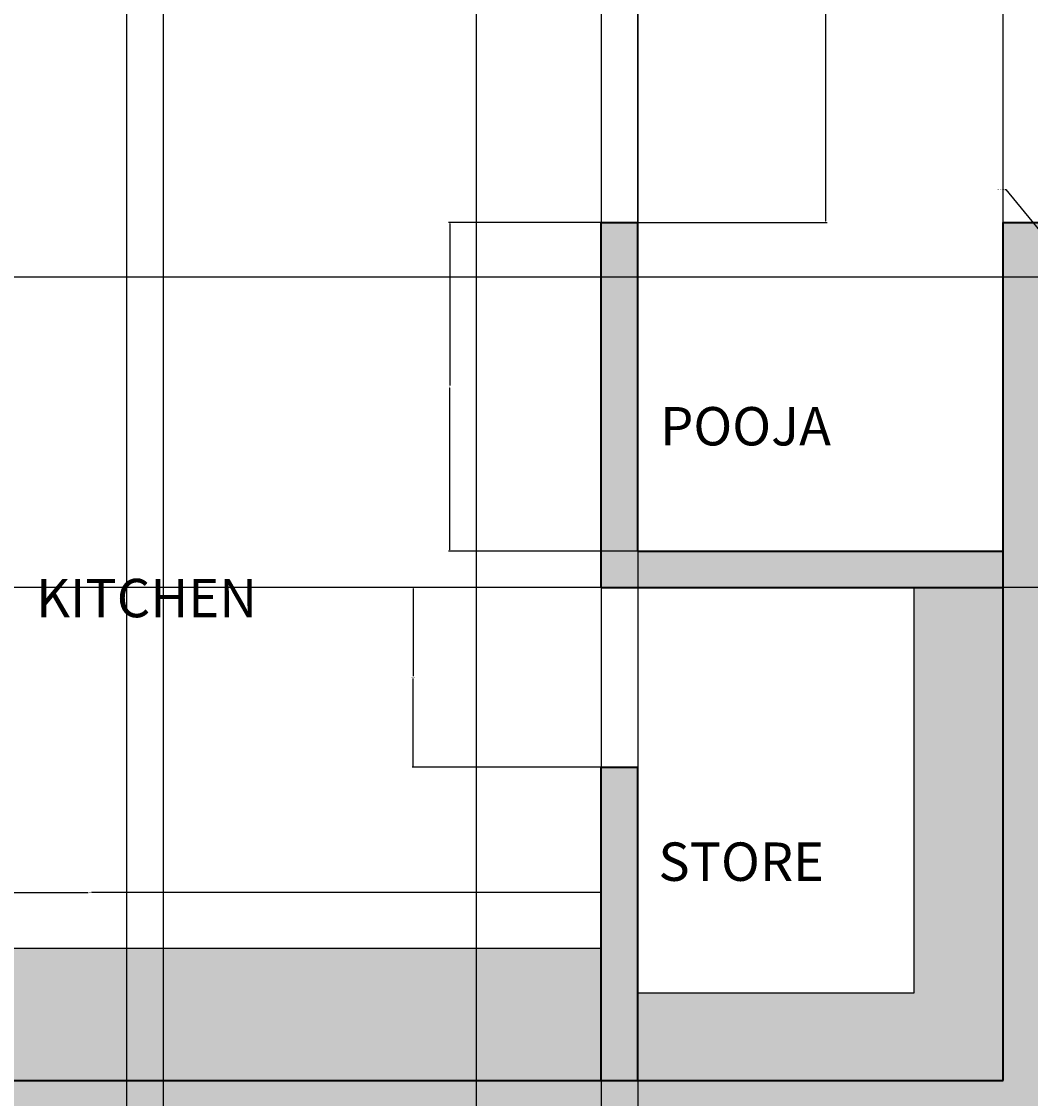
# Model space of a CAD drawing. Units: inches. Extents: x 2549 to 3108, y 1683 to 2362.
# Tile 3 of 30: x 2711 to 2877, y 1802 to 1979. Entities that reach past the tile are written whole.
import ezdxf

# ---------------------------------------------------------------- set-up
doc = ezdxf.new("R2010")
doc.units = ezdxf.units.IN
for name, color, linetype, lineweight in [('A-ANNO-DIMS', 2, 'Continuous', 18), ('A-AREA-IDEN', 7, 'Continuous', 18), ('A-FLOR-CASE', 8, 'Continuous', 25), ('A-FLOR-CASE-PATT', 42, 'Continuous', 13), ('A-FURN-PATT', 9, 'Continuous', 13), ('A-WALL', 7, 'Continuous', 35), ('A-WALL-PATT', 89, 'Continuous', 13)]:
    doc.layers.add(name, color=color, linetype=linetype, lineweight=lineweight)
doc.layers.add('C-PKNG-VEHI-PATT', color=251, linetype='Continuous', lineweight=13, true_color=0x636466)
doc.layers.add('C-PVMT-PATT', color=9, linetype='Continuous', lineweight=13, true_color=0xc7c8ca)
doc.styles.get("Standard").update_dxf_attribs({"font": 'arial.ttf'})
doc.dimstyles.get("Standard").update_dxf_attribs({"dimtxt": 0.18, "dimasz": 0.18, "dimexe": 0.18, "dimexo": 0.0625, "dimgap": 0.09, "dimtad": 0, "dimtih": 1, "dimtoh": 1, "dimdec": 4, "dimzin": 0, "dimdsep": 46, "dimtxsty": 'Standard', "dimcen": 0.09, "dimadec": 0, "dimazin": 0, "dimtfac": 1, "dimtdec": 4, "dimtofl": 0, "dimtmove": 0, "dimatfit": 3, "dimfxl": 1, "dimtolj": 1, "dimtzin": 0, "dimarcsym": 0})

# ---------------------------------------------------------------- blocks, each defined once
blk = doc.blocks.new('*D42')
at = {"layer": 'A-ANNO-DIMS', "color": 0, "lineweight": -2, "transparency": 16777216}
for p, q in [((2638.64, 2080.46), (2638.64, 1683.44)), ((2728.64, 2080.46), (2728.64, 1683.44)), ((2638.82, 1683.62), (2683.42, 1683.62)), ((2728.46, 1683.62), (2683.86, 1683.62))]:
    blk.add_line(p, q, dxfattribs=at)
at = {"layer": 'A-ANNO-DIMS', "color": 0, "transparency": 16777216}
for points in [[(2638.82, 1683.65), (2638.82, 1683.59), (2638.64, 1683.62)], [(2728.46, 1683.65), (2728.46, 1683.59), (2728.64, 1683.62)]]:
    blk.add_solid(points, dxfattribs=at)
at = {"layer": 'Defpoints', "color": 0, "transparency": 16777216}
for p in [(2638.64, 2080.52), (2728.64, 2080.52), (2728.64, 1683.62)]:
    blk.add_point(p, dxfattribs=at)
at = {"layer": 'A-ANNO-DIMS', "color": 0, "transparency": 16777216, "insert": (2683.64, 1683.62), "char_height": 0.18, "attachment_point": 5}
blk.add_mtext('\\A1;90', dxfattribs=at)
blk = doc.blocks.new('*D43')
at = {"layer": 'A-ANNO-DIMS', "color": 0, "lineweight": -2, "transparency": 16777216}
for p, q in [((2734.64, 2080.46), (2734.64, 1683.44)), ((2806.64, 2080.46), (2806.64, 1683.44)), ((2734.82, 1683.62), (2770.43, 1683.62)), ((2806.46, 1683.62), (2770.86, 1683.62))]:
    blk.add_line(p, q, dxfattribs=at)
at = {"layer": 'A-ANNO-DIMS', "color": 0, "transparency": 16777216}
for points in [[(2734.82, 1683.65), (2734.82, 1683.59), (2734.64, 1683.62)], [(2806.46, 1683.65), (2806.46, 1683.59), (2806.64, 1683.62)]]:
    blk.add_solid(points, dxfattribs=at)
at = {"layer": 'Defpoints', "color": 0, "transparency": 16777216}
for p in [(2734.64, 2080.52), (2806.64, 2080.52), (2806.64, 1683.62)]:
    blk.add_point(p, dxfattribs=at)
at = {"layer": 'A-ANNO-DIMS', "color": 0, "transparency": 16777216, "insert": (2770.64, 1683.62), "char_height": 0.18, "attachment_point": 5}
blk.add_mtext('\\A1;72', dxfattribs=at)
blk = doc.blocks.new('*D44')
at = {"layer": 'A-ANNO-DIMS', "color": 0, "lineweight": -2, "transparency": 16777216}
for p, q in [((2662.64, 2040.99), (2662.64, 1683.44)), ((2806.64, 2016.13), (2806.64, 1683.44)), ((2662.82, 1683.62), (2734.36, 1683.62)), ((2806.46, 1683.62), (2734.92, 1683.62))]:
    blk.add_line(p, q, dxfattribs=at)
at = {"layer": 'A-ANNO-DIMS', "color": 0, "transparency": 16777216}
for points in [[(2662.82, 1683.65), (2662.82, 1683.59), (2662.64, 1683.62)], [(2806.46, 1683.65), (2806.46, 1683.59), (2806.64, 1683.62)]]:
    blk.add_solid(points, dxfattribs=at)
at = {"layer": 'Defpoints', "color": 0, "transparency": 16777216}
for p in [(2662.64, 2041.06), (2806.64, 2016.19), (2806.64, 1683.62)]:
    blk.add_point(p, dxfattribs=at)
at = {"layer": 'A-ANNO-DIMS', "color": 0, "transparency": 16777216, "insert": (2734.64, 1683.62), "char_height": 0.18, "attachment_point": 5}
blk.add_mtext('\\A1;144', dxfattribs=at)
blk = doc.blocks.new('*D46')
at = {"layer": 'A-ANNO-DIMS', "color": 0, "lineweight": -2, "transparency": 16777216}
for p, q in [((2812.64, 2140.46), (2812.64, 1683.44)), ((3034.64, 2134.46), (3034.64, 1683.44)), ((2812.82, 1683.62), (2923.35, 1683.62)), ((3034.46, 1683.62), (2923.93, 1683.62))]:
    blk.add_line(p, q, dxfattribs=at)
at = {"layer": 'A-ANNO-DIMS', "color": 0, "transparency": 16777216}
for points in [[(2812.82, 1683.65), (2812.82, 1683.59), (2812.64, 1683.62)], [(3034.46, 1683.65), (3034.46, 1683.59), (3034.64, 1683.62)]]:
    blk.add_solid(points, dxfattribs=at)
at = {"layer": 'Defpoints', "color": 0, "transparency": 16777216}
for p in [(2812.64, 2140.52), (3034.64, 2134.52), (3034.64, 1683.62)]:
    blk.add_point(p, dxfattribs=at)
at = {"layer": 'A-ANNO-DIMS', "color": 0, "transparency": 16777216, "insert": (2923.64, 1683.62), "char_height": 0.18, "attachment_point": 5}
blk.add_mtext('\\A1;222', dxfattribs=at)
blk = doc.blocks.new('*D48')
at = {"layer": 'A-ANNO-DIMS', "color": 0, "lineweight": -2, "transparency": 16777216}
for p, q in [((2812.71, 2016.19), (2843.72, 2016.19)), ((2843.54, 2016.01), (2843.54, 1981.04)), ((2843.54, 1945.7), (2843.54, 1980.68)), ((2812.71, 1945.52), (2843.72, 1945.52))]:
    blk.add_line(p, q, dxfattribs=at)
at = {"layer": 'A-ANNO-DIMS', "color": 0, "transparency": 16777216}
for points in [[(2843.51, 2016.01), (2843.57, 2016.01), (2843.54, 2016.19)], [(2843.51, 1945.7), (2843.57, 1945.7), (2843.54, 1945.52)]]:
    blk.add_solid(points, dxfattribs=at)
at = {"layer": 'Defpoints', "color": 0, "transparency": 16777216}
for p in [(2812.64, 2016.19), (2812.64, 1945.52), (2843.54, 1945.52)]:
    blk.add_point(p, dxfattribs=at)
at = {"layer": 'A-ANNO-DIMS', "color": 0, "transparency": 16777216, "insert": (2843.54, 1980.86), "char_height": 0.18, "attachment_point": 5}
blk.add_mtext('\\A1;70.67', dxfattribs=at)
blk = doc.blocks.new('*D49')
at = {"layer": 'A-ANNO-DIMS', "color": 0, "lineweight": -2, "transparency": 16777216}
for p, q in [((2638.64, 1804.59), (2638.64, 1835.6)), ((2638.82, 1835.42), (2722.36, 1835.42)), ((2806.46, 1835.42), (2722.92, 1835.42)), ((2806.64, 1804.59), (2806.64, 1835.6))]:
    blk.add_line(p, q, dxfattribs=at)
at = {"layer": 'A-ANNO-DIMS', "color": 0, "transparency": 16777216}
for points in [[(2638.82, 1835.45), (2638.82, 1835.39), (2638.64, 1835.42)], [(2806.46, 1835.45), (2806.46, 1835.39), (2806.64, 1835.42)]]:
    blk.add_solid(points, dxfattribs=at)
at = {"layer": 'Defpoints', "color": 0, "transparency": 16777216}
for p in [(2806.64, 1835.42), (2638.64, 1804.52), (2806.64, 1804.52)]:
    blk.add_point(p, dxfattribs=at)
at = {"layer": 'A-ANNO-DIMS', "color": 0, "transparency": 16777216, "insert": (2722.64, 1835.42), "char_height": 0.18, "attachment_point": 5}
blk.add_mtext('\\A1;168', dxfattribs=at)
blk = doc.blocks.new('*D52')
at = {"layer": 'A-ANNO-DIMS', "color": 0, "lineweight": -2, "transparency": 16777216}
for p, q in [((2812.64, 1891.59), (2812.64, 2362.32)), ((2872.64, 1891.59), (2872.64, 2362.32)), ((2812.82, 2362.14), (2842.42, 2362.14)), ((2872.46, 2362.14), (2842.86, 2362.14))]:
    blk.add_line(p, q, dxfattribs=at)
at = {"layer": 'A-ANNO-DIMS', "color": 0, "transparency": 16777216}
for points in [[(2812.82, 2362.17), (2812.82, 2362.11), (2812.64, 2362.14)], [(2872.46, 2362.17), (2872.46, 2362.11), (2872.64, 2362.14)]]:
    blk.add_solid(points, dxfattribs=at)
at = {"layer": 'Defpoints', "color": 0, "transparency": 16777216}
for p in [(2872.64, 2362.14), (2812.64, 1891.52), (2872.64, 1891.52)]:
    blk.add_point(p, dxfattribs=at)
at = {"layer": 'A-ANNO-DIMS', "color": 0, "transparency": 16777216, "insert": (2842.64, 2362.14), "char_height": 0.18, "attachment_point": 5}
blk.add_mtext('\\A1;60', dxfattribs=at)
blk = doc.blocks.new('*D53')
at = {"layer": 'A-ANNO-DIMS', "color": 0, "lineweight": -2, "transparency": 16777216}
for p, q in [((2812.58, 1945.52), (2781.56, 1945.52)), ((2781.74, 1945.34), (2781.74, 1918.71)), ((2781.74, 1891.7), (2781.74, 1918.34)), ((2812.58, 1891.52), (2781.56, 1891.52))]:
    blk.add_line(p, q, dxfattribs=at)
at = {"layer": 'A-ANNO-DIMS', "color": 0, "transparency": 16777216}
for points in [[(2781.71, 1945.34), (2781.77, 1945.34), (2781.74, 1945.52)], [(2781.71, 1891.7), (2781.77, 1891.7), (2781.74, 1891.52)]]:
    blk.add_solid(points, dxfattribs=at)
at = {"layer": 'Defpoints', "color": 0, "transparency": 16777216}
for p in [(2781.74, 1945.52), (2812.64, 1945.52), (2812.64, 1891.52)]:
    blk.add_point(p, dxfattribs=at)
at = {"layer": 'A-ANNO-DIMS', "color": 0, "transparency": 16777216, "insert": (2781.74, 1918.52), "char_height": 0.18, "attachment_point": 5}
blk.add_mtext('\\A1;54', dxfattribs=at)
blk = doc.blocks.new('*D54')
at = {"layer": 'A-ANNO-DIMS', "color": 0, "lineweight": -2, "transparency": 16777216}
for p, q in [((2806.58, 1885.52), (2775.56, 1885.52)), ((2775.74, 1885.34), (2775.74, 1870.94)), ((2775.74, 1856.17), (2775.74, 1870.57)), ((2806.58, 1855.99), (2775.56, 1855.99))]:
    blk.add_line(p, q, dxfattribs=at)
at = {"layer": 'A-ANNO-DIMS', "color": 0, "transparency": 16777216}
for points in [[(2775.71, 1885.34), (2775.77, 1885.34), (2775.74, 1885.52)], [(2775.71, 1856.17), (2775.77, 1856.17), (2775.74, 1855.99)]]:
    blk.add_solid(points, dxfattribs=at)
at = {"layer": 'Defpoints', "color": 0, "transparency": 16777216}
for p in [(2775.74, 1885.52), (2806.64, 1885.52), (2806.64, 1855.99)]:
    blk.add_point(p, dxfattribs=at)
at = {"layer": 'A-ANNO-DIMS', "color": 0, "transparency": 16777216, "insert": (2775.74, 1870.75), "char_height": 0.18, "attachment_point": 5}
blk.add_mtext('\\A1;29.54', dxfattribs=at)
blk = doc.blocks.new('*D55')
at = {"layer": 'A-ANNO-DIMS', "color": 0, "lineweight": -2, "transparency": 16777216}
for p, q in [((2872.58, 1885.52), (2549.42, 1885.52)), ((2549.6, 1885.34), (2549.6, 1845.21)), ((2549.6, 1804.7), (2549.6, 1844.84)), ((2872.58, 1804.52), (2549.42, 1804.52))]:
    blk.add_line(p, q, dxfattribs=at)
at = {"layer": 'A-ANNO-DIMS', "color": 0, "transparency": 16777216}
for points in [[(2549.57, 1885.34), (2549.63, 1885.34), (2549.6, 1885.52)], [(2549.57, 1804.7), (2549.63, 1804.7), (2549.6, 1804.52)]]:
    blk.add_solid(points, dxfattribs=at)
at = {"layer": 'Defpoints', "color": 0, "transparency": 16777216}
for p in [(2549.6, 1885.52), (2872.64, 1885.52), (2872.64, 1804.52)]:
    blk.add_point(p, dxfattribs=at)
at = {"layer": 'A-ANNO-DIMS', "color": 0, "transparency": 16777216, "insert": (2549.6, 1845.02), "char_height": 0.18, "attachment_point": 5}
blk.add_mtext('\\A1;81', dxfattribs=at)
blk = doc.blocks.new('*D56')
at = {"layer": 'A-ANNO-DIMS', "color": 0, "lineweight": -2, "transparency": 16777216}
for p, q in [((3043.58, 1936.52), (2549.42, 1936.52)), ((2549.6, 1936.34), (2549.6, 1911.21)), ((2549.6, 1885.7), (2549.6, 1910.84)), ((3043.58, 1885.52), (2549.42, 1885.52))]:
    blk.add_line(p, q, dxfattribs=at)
at = {"layer": 'A-ANNO-DIMS', "color": 0, "transparency": 16777216}
for points in [[(2549.57, 1936.34), (2549.63, 1936.34), (2549.6, 1936.52)], [(2549.57, 1885.7), (2549.63, 1885.7), (2549.6, 1885.52)]]:
    blk.add_solid(points, dxfattribs=at)
at = {"layer": 'Defpoints', "color": 0, "transparency": 16777216}
for p in [(2549.6, 1936.52), (3043.64, 1936.52), (3043.64, 1885.52)]:
    blk.add_point(p, dxfattribs=at)
at = {"layer": 'A-ANNO-DIMS', "color": 0, "transparency": 16777216, "insert": (2549.6, 1911.02), "char_height": 0.18, "attachment_point": 5}
blk.add_mtext('\\A1;51', dxfattribs=at)
blk = doc.blocks.new('*D59')
at = {"layer": 'A-ANNO-DIMS', "color": 0, "lineweight": -2, "transparency": 16777216}
for p, q in [((2680.98, 1761.59), (2680.98, 2362.32)), ((2786.16, 1761.59), (2786.16, 2362.32)), ((2681.16, 2362.14), (2733.11, 2362.14)), ((2785.98, 2362.14), (2734.02, 2362.14))]:
    blk.add_line(p, q, dxfattribs=at)
at = {"layer": 'A-ANNO-DIMS', "color": 0, "transparency": 16777216}
for points in [[(2681.16, 2362.17), (2681.16, 2362.11), (2680.98, 2362.14)], [(2785.98, 2362.17), (2785.98, 2362.11), (2786.16, 2362.14)]]:
    blk.add_solid(points, dxfattribs=at)
at = {"layer": 'Defpoints', "color": 0, "transparency": 16777216}
for p in [(2786.16, 2362.14), (2680.98, 1761.52), (2786.16, 1761.52)]:
    blk.add_point(p, dxfattribs=at)
at = {"layer": 'A-ANNO-DIMS', "color": 0, "transparency": 16777216, "insert": (2733.57, 2362.14), "char_height": 0.18, "attachment_point": 5}
blk.add_mtext('\\A1;105.18', dxfattribs=at)
blk = doc.blocks.new('*D66')
at = {"layer": 'A-ANNO-DIMS', "color": 0, "lineweight": -2, "transparency": 16777216}
for p, q in [((2872.93, 1950.94), (2873.11, 1950.94)), ((2873.11, 1950.94), (2897.38, 1921.22)), ((2938.03, 1871.31), (2938.21, 1871.31)), ((2938.12, 1871.22), (2938.12, 1871.4))]:
    blk.add_line(p, q, dxfattribs=at)
at = {"layer": 'A-ANNO-DIMS', "color": 0, "transparency": 16777216}
blk.add_solid([(2897.4, 1921.24), (2897.36, 1921.2), (2897.49, 1921.08)], dxfattribs=at)
at = {"layer": 'Defpoints', "color": 0, "transparency": 16777216}
for p in [(2897.49, 1921.08), (2938.12, 1871.31)]:
    blk.add_point(p, dxfattribs=at)
at = {"layer": 'A-ANNO-DIMS', "color": 0, "transparency": 16777216, "insert": (2872.26, 1950.94), "char_height": 0.18, "attachment_point": 5}
blk.add_mtext('\\A1;2X R64.25', dxfattribs=at)

msp = doc.modelspace()

# ---------------------------------------------------------------- hatches: boundary and pattern name
at = {"layer": 'A-FLOR-CASE-PATT', "transparency": 33554539}
h = msp.add_hatch(color=256, dxfattribs=at)
h.dxf.hatch_style = 1
h.paths.add_polyline_path([(2664.8522, 1925.2912), (2638.6427, 1925.2912), (2638.6427, 1804.5237), (2662.6427, 1804.5237), (2806.6427, 1804.5237), (2806.6427, 1826.2821), (2664.8522, 1826.2821)])
h.paths.add_polyline_path([(2872.6427, 1885.5237), (2858.0172, 1885.5237), (2858.0172, 1818.9517), (2812.6427, 1818.9517), (2812.6427, 1804.5237), (2872.6427, 1804.5237)])
at = {"layer": 'A-FURN-PATT', "transparency": 33554567}
h = msp.add_hatch(color=256, dxfattribs=at)
h.dxf.hatch_style = 1
h.paths.add_polyline_path([(2708.7147, 2271.6737), (2675.2813, 2271.6737), (2675.2813, 2262.0404), (2708.7147, 2262.0404)])
h.paths.add_polyline_path([(2980.8246, 2271.6737), (2947.3913, 2271.6737), (2947.3913, 2262.0404), (2980.8246, 2262.0404)])
h.paths.add_polyline_path([(2748.8496, 2101.6383), (2798.148, 2101.6383), (2798.148, 2111.4248), (2748.8496, 2111.4248)], flags=9)
h.paths.add_polyline_path([(2685.2081, 2101.489), (2719.3253, 2101.489), (2719.3253, 2111.2819), (2685.2081, 2111.2819)], flags=9)
h.paths.add_polyline_path([(2814.6852, 1907.1328), (2847.8384, 1907.1328), (2847.8384, 1916.9258), (2814.6852, 1916.9258)], flags=9)
h.paths.add_polyline_path([(2814.3906, 1835.5864), (2848.0172, 1835.5864), (2848.0172, 1845.3794), (2814.3906, 1845.3794)], flags=9)
h.paths.add_polyline_path([(2800.5245, 1759.1674), (2853.7435, 1759.1674), (2853.7435, 1768.954), (2800.5245, 1768.954)], flags=9)
h.paths.add_polyline_path([(2972.4611, 1807.3305), (3015.3943, 1807.3305), (3015.3943, 1817.117), (2972.4611, 1817.117)], flags=9)
h.paths.add_polyline_path([(2902.3327, 1888.6731), (2937.9131, 1888.6731), (2937.9131, 1898.4661), (2902.3327, 1898.4661)], flags=9)
h.paths.add_polyline_path([(2712.1779, 1878.9039), (2754.1257, 1878.9039), (2754.1257, 1888.6904), (2712.1779, 1888.6904)], flags=9)
h.paths.add_polyline_path([(2614.0056, 2012.812), (2650.0251, 2012.812), (2650.0251, 2022.4371), (2614.0056, 2022.4371)], flags=9)
h.paths.add_polyline_path([(2713.3129, 2003.1645), (2747.4237, 2003.1645), (2747.4237, 2012.951), (2713.3129, 2012.951)], flags=9)
h.paths.add_polyline_path([(2950.1379, 2001.6934), (2982.2992, 2001.6934), (2982.2992, 2011.48), (2950.1379, 2011.48)], flags=9)
h.paths.add_polyline_path([(2940.864, 2238.5537), (2997.5066, 2238.5537), (2997.5066, 2248.3466), (2940.864, 2248.3466)], flags=9)
h.paths.add_polyline_path([(2821.5457, 2202.8348), (2855.663, 2202.8348), (2855.663, 2212.6278), (2821.5457, 2212.6278)], flags=9)
h.paths.add_polyline_path([(2661.8026, 2238.6249), (2718.4451, 2238.6249), (2718.4451, 2248.4179), (2661.8026, 2248.4179)], flags=9)
h = msp.add_hatch(color=256, dxfattribs=at)
h.dxf.hatch_style = 1
h.paths.add_polyline_path([(2906.5064, 1905.2148), (2905.2584, 1904.3827), (2907.0611, 1900.7772), (2908.3092, 1901.6092)])
h.paths.add_polyline_path([(2936.522, 1914.8044), (2935.2739, 1915.6364), (2932.6391, 1912.5856), (2933.8871, 1911.7535)])
h.paths.add_polyline_path([(2950.2508, 1905.6518), (2949.0027, 1906.4839), (2947.1999, 1902.8783), (2948.448, 1902.0463)])
h.paths.add_polyline_path([(2958.5713, 1918.1326), (2956.9072, 1919.242), (2952.4696, 1908.98, 1.38742744), (2954.9657, 1907.3159)])
h.paths.add_polyline_path([(2945.2585, 1927.0078), (2943.5944, 1928.1172), (2934.9965, 1920.6287, 1.38742744), (2937.4927, 1918.9646)])
h.paths.add_polyline_path([(2748.8496, 2101.6383), (2798.148, 2101.6383), (2798.148, 2111.4248), (2748.8496, 2111.4248)], flags=9)
h.paths.add_polyline_path([(2685.2081, 2101.489), (2719.3253, 2101.489), (2719.3253, 2111.2819), (2685.2081, 2111.2819)], flags=9)
h.paths.add_polyline_path([(2814.6852, 1907.1328), (2847.8384, 1907.1328), (2847.8384, 1916.9258), (2814.6852, 1916.9258)], flags=9)
h.paths.add_polyline_path([(2814.3906, 1835.5864), (2848.0172, 1835.5864), (2848.0172, 1845.3794), (2814.3906, 1845.3794)], flags=9)
h.paths.add_polyline_path([(2800.5245, 1759.1674), (2853.7435, 1759.1674), (2853.7435, 1768.954), (2800.5245, 1768.954)], flags=9)
h.paths.add_polyline_path([(2972.4611, 1807.3305), (3015.3943, 1807.3305), (3015.3943, 1817.117), (2972.4611, 1817.117)], flags=9)
h.paths.add_polyline_path([(2902.3327, 1888.6731), (2937.9131, 1888.6731), (2937.9131, 1898.4661), (2902.3327, 1898.4661)], flags=9)
h.paths.add_polyline_path([(2712.1779, 1878.9039), (2754.1257, 1878.9039), (2754.1257, 1888.6904), (2712.1779, 1888.6904)], flags=9)
h.paths.add_polyline_path([(2614.0056, 2012.812), (2650.0251, 2012.812), (2650.0251, 2022.4371), (2614.0056, 2022.4371)], flags=9)
h.paths.add_polyline_path([(2713.3129, 2003.1645), (2747.4237, 2003.1645), (2747.4237, 2012.951), (2713.3129, 2012.951)], flags=9)
h.paths.add_polyline_path([(2950.1379, 2001.6934), (2982.2992, 2001.6934), (2982.2992, 2011.48), (2950.1379, 2011.48)], flags=9)
h.paths.add_polyline_path([(2940.864, 2238.5537), (2997.5066, 2238.5537), (2997.5066, 2248.3466), (2940.864, 2248.3466)], flags=9)
h.paths.add_polyline_path([(2821.5457, 2202.8348), (2855.663, 2202.8348), (2855.663, 2212.6278), (2821.5457, 2212.6278)], flags=9)
h.paths.add_polyline_path([(2661.8026, 2238.6249), (2718.4451, 2238.6249), (2718.4451, 2248.4179), (2661.8026, 2248.4179)], flags=9)
at = {"layer": 'A-WALL-PATT'}
h = msp.add_hatch(color=256, dxfattribs=at)
h.dxf.hatch_style = 1
h.paths.add_polyline_path([(2638.6427, 2272.5237), (3034.6427, 2272.5237), (3034.6427, 1936.5237), (3043.6427, 1936.5237), (3043.6427, 2281.5237), (2629.6427, 2281.5237), (2629.6427, 2074.5237), (2812.6427, 2074.5237), (2812.6427, 2140.5237), (2785.7177, 2140.5237), (2785.7177, 2134.5237), (2806.6427, 2134.5237), (2806.6427, 2080.5237), (2638.6427, 2080.5237)])
h.paths.add_polyline_path([(2638.6427, 1972.5237), (2662.6427, 1972.5237), (2662.6427, 2041.0557), (2653.6427, 2041.0557), (2653.6427, 1978.5237), (2629.6427, 1978.5237), (2629.6427, 1795.5237), (2662.6427, 1795.5237), (2881.6427, 1795.5237), (2881.6427, 1936.5237), (2965.9351, 1936.5237), (2965.9351, 1974.5439), (2959.9351, 1974.5439), (2959.9351, 1945.5237), (2881.6427, 1945.5237), (2872.6427, 1945.5237), (2872.6427, 1804.5237), (2662.6427, 1804.5237), (2638.6427, 1804.5237)])
h = msp.add_hatch(color=256, dxfattribs=at)
h.dxf.hatch_style = 1
h.paths.add_polyline_path([(2747.213, 2140.5237), (2638.6427, 2140.5237), (2638.6427, 2134.5237), (2747.213, 2134.5237)])
h.paths.add_polyline_path([(2734.6427, 2109.4935), (2728.6427, 2109.4935), (2728.6427, 2080.5237), (2734.6427, 2080.5237)])
h.paths.add_polyline_path([(2812.6427, 2074.5237), (2806.6427, 2074.5237), (2806.6427, 2016.1911), (2812.6427, 2016.1911)])
h.paths.add_polyline_path([(2812.6427, 1945.5237), (2806.6427, 1945.5237), (2806.6427, 1885.5237), (2872.6427, 1885.5237), (2872.6427, 1891.5237), (2812.6427, 1891.5237)])
h.paths.add_polyline_path([(2812.6427, 1855.9859), (2806.6427, 1855.9859), (2806.6427, 1804.5237), (2812.6427, 1804.5237)])
at = {"layer": 'C-PKNG-VEHI-PATT'}
h = msp.add_hatch(color=256, dxfattribs=at)
h.dxf.hatch_style = 1
edge = h.paths.add_edge_path()
edge.add_ellipse((2935.7258, 1791.964), major_axis=(-50.66, 0), ratio=0.84230387, start_angle=248.165046, end_angle=265.722579)
edge.add_line((2938.911, 1834.5507), (2925.8653, 1834.5507))
edge.add_ellipse((2929.0505, 1791.964), major_axis=(50.66, 0), ratio=0.84230387, start_angle=94.277421, end_angle=111.834954)
edge.add_line((2912.8508, 1832.3947), (2914.2044, 1822.2495))
edge.add_ellipse((2930.6538, 1783.1023), major_axis=(-49.3014, 0), ratio=0.84230387, start_angle=-85.12993, end_angle=-67.208085, ccw=False)
edge.add_line((2927.1247, 1824.5225), (2937.6516, 1824.5225))
edge.add_ellipse((2934.1225, 1783.1023), major_axis=(49.3014, 0), ratio=0.84230387, start_angle=67.208085, end_angle=85.12993, ccw=False)
edge.add_line((2950.5719, 1822.2495), (2951.9255, 1832.3947))
edge = h.paths.add_edge_path()
edge.add_ellipse((2903.4793, 1857.3351), major_axis=(-34.7979, 0), ratio=0.84230387, start_angle=180, end_angle=209.43857)
edge.add_ellipse((2961.297, 1857.3351), major_axis=(34.7979, 0), ratio=0.84230387, start_angle=150.56143, end_angle=180)
edge.add_line((2926.4991, 1857.3351), (2926.4991, 1843.7609))
edge.add_ellipse((2924.1251, 1844.3143), major_axis=(-0.2209, 3.9278), ratio=0.60383358, start_angle=89.002014, end_angle=253.657408, ccw=False)
edge.add_line((2921.7512, 1844.2222), (2921.7512, 1853.3975))
edge.add_line((2921.7512, 1853.3975), (2925.269, 1855.8484))
edge.add_ellipse((2925.4782, 1855.4931), major_axis=(0.4584, 0), ratio=0.84230387, start_angle=90, end_angle=134.480211, ccw=False)
edge.add_line((2925.4782, 1855.8792), (2926.4991, 1855.8792))
edge.add_line((2926.4991, 1855.8792), (2926.4991, 1857.3351))
edge.add_ellipse((2961.297, 1857.3351), major_axis=(34.7979, 0), ratio=0.84230387, start_angle=150.56143, end_angle=180, ccw=False)
edge.add_line((2932.3882, 1873.6501), (2932.3882, 1875.7801))
edge.add_ellipse((2932.3882, 1875.3939), major_axis=(0.4584, 0), ratio=0.84230387, start_angle=90, end_angle=127.93313)
edge.add_line((2932.1366, 1875.7167), (2928.5915, 1873.7564))
edge.add_ellipse((2899.9271, 2002.4692), major_axis=(155.4756, 0), ratio=0.84230387, start_angle=-80.743434, end_angle=-77.445067, ccw=False)
edge.add_ellipse((2949.4402, 1715.2151), major_axis=(-189.1422, 0), ratio=0.84230387, start_angle=-79.790461, end_angle=-77.555373)
edge.add_ellipse((3300.3614, 1852.5642), major_axis=(-386.1662, 0), ratio=0.84230387, start_angle=-2.863715, end_angle=2.198541)
edge.add_ellipse((2929.0505, 1792.5159), major_axis=(-55.6192, 0), ratio=0.84230387, start_angle=-85.917589, end_angle=-72.280047, ccw=False)
edge.add_line((2925.7129, 1839.2798), (2939.0634, 1839.2798))
edge.add_ellipse((2935.7258, 1792.5159), major_axis=(55.6192, 0), ratio=0.84230387, start_angle=72.280047, end_angle=85.917589, ccw=False)
edge.add_ellipse((2564.4149, 1852.5642), major_axis=(-386.1662, 0), ratio=0.84230387, start_angle=177.801459, end_angle=182.863715)
edge.add_ellipse((2915.3361, 1715.2151), major_axis=(189.1422, 0), ratio=0.84230387, start_angle=77.555373, end_angle=79.790461)
edge.add_ellipse((2964.8492, 2002.4692), major_axis=(-155.4756, 0), ratio=0.84230387, start_angle=77.445067, end_angle=80.743434, ccw=False)
edge.add_line((2936.1848, 1873.7564), (2932.6397, 1875.7167))
edge.add_ellipse((2932.3882, 1875.3939), major_axis=(0.4584, 0), ratio=0.84230387, start_angle=52.06687, end_angle=90)
edge.add_line((2932.3882, 1875.7801), (2932.3882, 1873.6501))
edge.add_ellipse((2903.4793, 1857.3351), major_axis=(-34.7979, 0), ratio=0.84230387, start_angle=180, end_angle=209.43857, ccw=False)
edge.add_line((2938.2772, 1857.3351), (2938.2772, 1855.8792))
edge.add_line((2938.2772, 1855.8792), (2939.4059, 1855.8792))
edge.add_ellipse((2939.2981, 1855.4931), major_axis=(-0.4584, 0), ratio=0.84230387, start_angle=225.519789, end_angle=270, ccw=False)
edge.add_line((2939.5903, 1855.7906), (2943.0251, 1853.3975))
edge.add_line((2943.0251, 1853.3975), (2943.0251, 1844.2222))
edge.add_ellipse((2940.6512, 1844.3143), major_axis=(0.2209, 3.9278), ratio=0.60383358, start_angle=106.342592, end_angle=270.997986, ccw=False)
edge.add_line((2938.2772, 1843.7609), (2938.2772, 1857.3351))
edge = h.paths.add_edge_path()
edge.add_ellipse((2932.3882, 1865.1973), major_axis=(91.081, 0), ratio=0.84230387, start_angle=256.401865, end_angle=283.598135, ccw=False)
edge.add_line((2914.2044, 1790.0239), (2914.2044, 1778.3622))
edge.add_ellipse((2932.3882, 1853.5356), major_axis=(91.081, 0), ratio=0.84230387, start_angle=256.401865, end_angle=283.598135)
edge.add_line((2950.5719, 1778.3622), (2950.5719, 1790.0239))
edge = h.paths.add_edge_path()
edge.add_ellipse((2948.7383, 1772.3145), major_axis=(1.8336, 0), ratio=0.84230387, start_angle=0, end_angle=90)
edge.add_line((2948.7383, 1773.859), (2916.038, 1773.859))
edge.add_ellipse((2916.038, 1772.3145), major_axis=(1.8336, 0), ratio=0.84230387, start_angle=90, end_angle=180)
edge.add_line((2914.2044, 1772.3145), (2914.2044, 1760.2558))
edge.add_line((2914.2044, 1760.2558), (2950.5719, 1760.2558))
edge.add_line((2950.5719, 1760.2558), (2950.5719, 1772.3145))
h.paths.add_polyline_path([(2748.8496, 2101.6383), (2798.148, 2101.6383), (2798.148, 2111.4248), (2748.8496, 2111.4248)], flags=9)
h.paths.add_polyline_path([(2685.2081, 2101.489), (2719.3253, 2101.489), (2719.3253, 2111.2819), (2685.2081, 2111.2819)], flags=9)
h.paths.add_polyline_path([(2814.6852, 1907.1328), (2847.8384, 1907.1328), (2847.8384, 1916.9258), (2814.6852, 1916.9258)], flags=9)
h.paths.add_polyline_path([(2814.3906, 1835.5864), (2848.0172, 1835.5864), (2848.0172, 1845.3794), (2814.3906, 1845.3794)], flags=9)
h.paths.add_polyline_path([(2800.5245, 1759.1674), (2853.7435, 1759.1674), (2853.7435, 1768.954), (2800.5245, 1768.954)], flags=9)
h.paths.add_polyline_path([(2972.4611, 1807.3305), (3015.3943, 1807.3305), (3015.3943, 1817.117), (2972.4611, 1817.117)], flags=9)
h.paths.add_polyline_path([(2902.3327, 1888.6731), (2937.9131, 1888.6731), (2937.9131, 1898.4661), (2902.3327, 1898.4661)], flags=9)
h.paths.add_polyline_path([(2712.1779, 1878.9039), (2754.1257, 1878.9039), (2754.1257, 1888.6904), (2712.1779, 1888.6904)], flags=9)
h.paths.add_polyline_path([(2614.0056, 2012.812), (2650.0251, 2012.812), (2650.0251, 2022.4371), (2614.0056, 2022.4371)], flags=9)
h.paths.add_polyline_path([(2713.3129, 2003.1645), (2747.4237, 2003.1645), (2747.4237, 2012.951), (2713.3129, 2012.951)], flags=9)
h.paths.add_polyline_path([(2950.1379, 2001.6934), (2982.2992, 2001.6934), (2982.2992, 2011.48), (2950.1379, 2011.48)], flags=9)
h.paths.add_polyline_path([(2940.864, 2238.5537), (2997.5066, 2238.5537), (2997.5066, 2248.3466), (2940.864, 2248.3466)], flags=9)
h.paths.add_polyline_path([(2821.5457, 2202.8348), (2855.663, 2202.8348), (2855.663, 2212.6278), (2821.5457, 2212.6278)], flags=9)
h.paths.add_polyline_path([(2661.8026, 2238.6249), (2718.4451, 2238.6249), (2718.4451, 2248.4179), (2661.8026, 2248.4179)], flags=9)
at = {"layer": 'C-PVMT-PATT'}
h = msp.add_hatch(color=256, dxfattribs=at)
h.dxf.hatch_style = 1
h.paths.add_polyline_path([(3067.6427, 2305.5237), (2605.6427, 2305.5237), (2605.6427, 2074.5237), (2629.6427, 2074.5237), (2629.6427, 2281.5237), (3043.6427, 2281.5237), (3043.6427, 1885.5237), (3043.6427, 1872.8745), (3031.1672, 1872.8745), (3031.1672, 1862.5731), (2995.8054, 1862.5731), (2995.8054, 1872.8745), (2983.1752, 1872.8745), (2983.1752, 1885.5237), (2881.6427, 1885.5237), (2881.6427, 1795.5237), (2751.0977, 1795.5237), (2751.0977, 1761.5237), (2786.1577, 1761.5237), (2786.1577, 1723.5237), (2881.84, 1723.5237), (2881.84, 1714.5237), (3067.6427, 1714.5237), (3067.6427, 1723.5237)])
edge = h.paths.add_edge_path(flags=16)
edge.add_ellipse((2949.4402, 1710.9683), major_axis=(-194.1014, 0), ratio=0.84230387, start_angle=-77.874034, end_angle=-76.219471, ccw=False)
edge.add_ellipse((2949.4402, 1715.2151), major_axis=(-189.1422, 0), ratio=0.84230387, start_angle=-79.790461, end_angle=-77.555373, ccw=False)
edge.add_ellipse((2899.9271, 2002.4692), major_axis=(155.4756, 0), ratio=0.84230387, start_angle=-80.743434, end_angle=-77.445067)
edge.add_line((2928.5915, 1873.7564), (2932.3882, 1875.8558))
edge.add_line((2932.3882, 1875.8558), (2936.1848, 1873.7564))
edge.add_ellipse((2964.8492, 2002.4692), major_axis=(-155.4756, 0), ratio=0.84230387, start_angle=77.445067, end_angle=80.743434)
edge.add_ellipse((2915.3361, 1715.2151), major_axis=(189.1422, 0), ratio=0.84230387, start_angle=77.555373, end_angle=79.790461, ccw=False)
edge.add_ellipse((2915.3361, 1710.9683), major_axis=(-194.1014, 0), ratio=0.84230387, start_angle=256.219471, end_angle=257.874034, ccw=False)
edge.add_ellipse((2628.2871, 1850.2612), major_axis=(-327.2532, 0), ratio=0.84230387, start_angle=182.17995, end_angle=183.650428, ccw=False)
edge.add_ellipse((2955.5637, 1861.9334), major_axis=(-0.9168, 0), ratio=0.84230387, start_angle=180, end_angle=270, ccw=False)
edge.add_line((2956.4805, 1862.3857), (2956.4805, 1846.4866))
edge.add_ellipse((2955.5637, 1846.939), major_axis=(-0.9168, 0), ratio=0.84230387, start_angle=90, end_angle=180, ccw=False)
edge.add_ellipse((-3607.0606, 1835.832), major_axis=(-6562.6242, 0), ratio=0.84230387, start_angle=179.61613322, end_angle=180.09022909, ccw=False)
edge.add_ellipse((2955.5637, 1791.0926), major_axis=(0.9168, 0), ratio=0.84230387, start_angle=0, end_angle=90, ccw=False)
edge.add_line((2956.4805, 1791.545), (2956.4805, 1775.6459))
edge.add_ellipse((2955.5637, 1776.0982), major_axis=(0.9168, 0), ratio=0.84230387, start_angle=270, end_angle=360, ccw=False)
edge.add_ellipse((-3607.0606, 1835.832), major_axis=(-6562.6242, 0), ratio=0.84230387, start_angle=179.3813568, end_angle=179.47172853, ccw=False)
edge.add_ellipse((2954.5907, 1763.8768), major_axis=(-1.3752, 0), ratio=0.84230387, start_angle=179.371763, end_angle=248.464757, ccw=False)
edge.add_ellipse((-3607.519, 1835.832), major_axis=(-6564.0409, 0), ratio=0.842303863, start_angle=179.35344594, end_angle=179.37176282, ccw=False)
edge.add_ellipse((2952.6829, 1761.8002), major_axis=(3.2503, 0), ratio=0.84230387, start_angle=-90, end_angle=-0.646554, ccw=False)
edge.add_line((2952.6829, 1759.0625), (2912.0934, 1759.0625))
edge.add_ellipse((2912.0934, 1761.8002), major_axis=(3.2503, 0), ratio=0.84230387, start_angle=180.646554, end_angle=270, ccw=False)
edge.add_ellipse((9472.2953, 1835.832), major_axis=(-6564.0409, 0), ratio=0.842303871, start_angle=0.62823722, end_angle=0.6465541, ccw=False)
edge.add_ellipse((2910.1856, 1763.8768), major_axis=(1.3752, 0), ratio=0.84230387, start_angle=111.535244, end_angle=180.628237, ccw=False)
edge.add_ellipse((9471.8369, 1835.832), major_axis=(-6562.6242, 0), ratio=0.84230387, start_angle=0.52827147, end_angle=0.6465541, ccw=False)
edge.add_ellipse((2909.2126, 1776.0982), major_axis=(-0.9168, 0), ratio=0.84230387, start_angle=0, end_angle=90, ccw=False)
edge.add_line((2908.2958, 1775.6459), (2908.2958, 1791.545))
edge.add_ellipse((2909.2126, 1791.0926), major_axis=(-0.9168, 0), ratio=0.84230387, start_angle=-90, end_angle=0, ccw=False)
edge.add_ellipse((9471.8369, 1835.832), major_axis=(-6562.6242, 0), ratio=0.84230387, start_angle=-0.09022909, end_angle=0.38386678, ccw=False)
edge.add_ellipse((2909.2126, 1846.939), major_axis=(-0.9168, 0), ratio=0.84230387, start_angle=0, end_angle=90, ccw=False)
edge.add_line((2908.2958, 1846.4866), (2908.2958, 1862.3857))
edge.add_ellipse((2909.2126, 1861.9334), major_axis=(0.9168, 0), ratio=0.84230387, start_angle=90, end_angle=180, ccw=False)
edge.add_ellipse((3236.4892, 1850.2612), major_axis=(327.2532, 0), ratio=0.84230387, start_angle=176.349572, end_angle=177.82005, ccw=False)
edge = h.paths.add_edge_path(flags=0)
edge.add_ellipse((2903.4793, 1857.3351), major_axis=(-34.7979, 0), ratio=0.84230387, start_angle=180, end_angle=209.43857, ccw=False)
edge.add_line((2938.2772, 1857.3351), (2938.2772, 1855.8792))
edge.add_line((2938.2772, 1855.8792), (2939.4631, 1855.8792))
edge.add_line((2939.4631, 1855.8792), (2943.0251, 1853.3975))
edge.add_line((2943.0251, 1853.3975), (2943.0251, 1844.2222))
edge.add_ellipse((2940.6512, 1844.3143), major_axis=(0.2209, 3.9278), ratio=0.60383358, start_angle=106.342592, end_angle=270.997986, ccw=False)
edge.add_line((2938.2772, 1843.7609), (2938.2772, 1857.3351))
edge.add_ellipse((2903.4793, 1857.3351), major_axis=(-34.7979, 0), ratio=0.84230387, start_angle=180, end_angle=209.43857)
edge.add_ellipse((2961.297, 1857.3351), major_axis=(34.7979, 0), ratio=0.84230387, start_angle=150.56143, end_angle=180)
edge.add_line((2926.4991, 1857.3351), (2926.4991, 1843.7609))
edge.add_ellipse((2924.1251, 1844.3143), major_axis=(-0.2209, 3.9278), ratio=0.60383358, start_angle=89.002014, end_angle=253.657408, ccw=False)
edge.add_line((2921.7512, 1844.2222), (2921.7512, 1853.3975))
edge.add_line((2921.7512, 1853.3975), (2925.3132, 1855.8792))
edge.add_line((2925.3132, 1855.8792), (2926.4991, 1855.8792))
edge.add_line((2926.4991, 1855.8792), (2926.4991, 1857.3351))
edge.add_ellipse((2961.297, 1857.3351), major_axis=(34.7979, 0), ratio=0.84230387, start_angle=150.56143, end_angle=180, ccw=False)
edge = h.paths.add_edge_path(flags=0)
edge.add_ellipse((2929.0505, 1791.964), major_axis=(50.66, 0), ratio=0.84230387, start_angle=94.277421, end_angle=111.834954, ccw=False)
edge.add_line((2925.8653, 1834.5507), (2938.911, 1834.5507))
edge.add_ellipse((2935.7258, 1791.964), major_axis=(-50.66, 0), ratio=0.84230387, start_angle=248.165046, end_angle=265.722579, ccw=False)
edge.add_line((2951.9255, 1832.3947), (2950.5719, 1822.2495))
edge.add_ellipse((2934.1225, 1783.1023), major_axis=(49.3014, 0), ratio=0.84230387, start_angle=67.208085, end_angle=85.12993)
edge.add_line((2937.6516, 1824.5225), (2927.1247, 1824.5225))
edge.add_ellipse((2930.6538, 1783.1023), major_axis=(-49.3014, 0), ratio=0.84230387, start_angle=-85.12993, end_angle=-67.208085)
edge.add_line((2914.2044, 1822.2495), (2912.8508, 1832.3947))
edge = h.paths.add_edge_path(flags=0)
edge.add_line((2910.1338, 1829.4651), (2912.6432, 1821.2711))
edge.add_ellipse((5203.7787, 1816.4367), major_axis=(-2291.1426, 0), ratio=0.84230387, start_angle=-0.1208974, end_angle=0.3640763)
edge.add_line((2912.7012, 1801.8782), (2910.3305, 1792.5698))
edge.add_ellipse((9471.8369, 1835.832), major_axis=(-6561.7074, 0), ratio=0.84230387, start_angle=0.05559431, end_angle=0.37776419, ccw=False)
edge = h.paths.add_edge_path(flags=0)
edge.add_ellipse((-3607.0606, 1835.832), major_axis=(6561.7074, 0), ratio=0.84230387, start_angle=-0.37776419, end_angle=-0.05559431, ccw=False)
edge.add_line((2954.4458, 1792.5698), (2952.0751, 1801.8782))
edge.add_ellipse((660.9976, 1816.4367), major_axis=(2291.1426, 0), ratio=0.84230387, start_angle=-0.3640763, end_angle=0.1208974)
edge.add_line((2952.1331, 1821.2711), (2954.6425, 1829.4651))
edge = h.paths.add_edge_path(flags=0)
edge.add_ellipse((2932.3882, 1865.1973), major_axis=(91.081, 0), ratio=0.84230387, start_angle=256.401865, end_angle=283.598135)
edge.add_line((2950.5719, 1790.0239), (2950.5719, 1778.3622))
edge.add_ellipse((2932.3882, 1853.5356), major_axis=(91.081, 0), ratio=0.84230387, start_angle=256.401865, end_angle=283.598135, ccw=False)
edge.add_line((2914.2044, 1778.3622), (2914.2044, 1790.0239))
edge = h.paths.add_edge_path(flags=0)
edge.add_line((2916.038, 1773.859), (2948.7383, 1773.859))
edge.add_ellipse((2948.7383, 1772.3145), major_axis=(1.8336, 0), ratio=0.84230387, start_angle=0, end_angle=90, ccw=False)
edge.add_line((2950.5719, 1772.3145), (2950.5719, 1760.2558))
edge.add_line((2950.5719, 1760.2558), (2914.2044, 1760.2558))
edge.add_line((2914.2044, 1760.2558), (2914.2044, 1772.3145))
edge.add_ellipse((2916.038, 1772.3145), major_axis=(1.8336, 0), ratio=0.84230387, start_angle=90, end_angle=180, ccw=False)
h.paths.add_polyline_path([(2629.6427, 1978.5237), (2605.6427, 1978.5237), (2605.6427, 1723.5237), (2629.6427, 1723.5237), (2629.6427, 1795.5237)], flags=17)
h.paths.add_polyline_path([(2800.5245, 1759.1674), (2853.7435, 1759.1674), (2853.7435, 1768.954), (2800.5245, 1768.954)], flags=24)
h.paths.add_polyline_path([(2972.4611, 1807.3305), (3015.3943, 1807.3305), (3015.3943, 1817.117), (2972.4611, 1817.117)], flags=24)

# ---------------------------------------------------------------- linework, layer by layer
at = {"layer": 'A-FLOR-CASE'}
for p, q in [((2858.0172, 1818.9517), (2858.0172, 1885.5237)), ((2664.8522, 1826.2821), (2806.6427, 1826.2821)), ((2812.6427, 1818.9517), (2812.6427, 1818.9517)), ((2812.6427, 1818.9517), (2858.0172, 1818.9517))]:
    msp.add_line(p, q, dxfattribs=at)
at = {"layer": 'A-WALL'}
for p, q in [((2806.6427, 1885.5237), (2806.6427, 1945.5237)), ((2812.6427, 1891.5237), (2812.6427, 1945.5237)), ((2872.6427, 1804.5237), (2872.6427, 1945.5237)), ((2806.6427, 1804.5237), (2806.6427, 1855.9859)), ((2806.6427, 1855.9859), (2812.6427, 1855.9859)), ((2812.6427, 1804.5237), (2812.6427, 1855.9859))]:
    msp.add_line(p, q, dxfattribs=at)
for points in [[(2806.6427, 1945.5237), (2812.6427, 1945.5237)], [(2872.6427, 1945.5237), (2881.6427, 1945.5237)], [(2812.6427, 1891.5237), (2872.6427, 1891.5237)], [(2806.6427, 1885.5237), (2872.6427, 1885.5237)], [(2638.6427, 1804.5237), (2662.6427, 1804.5237), (2872.6427, 1804.5237)]]:
    msp.add_lwpolyline(points, dxfattribs=at)

# ---------------------------------------------------------------- texts
at = {"layer": 'A-AREA-IDEN'}
for s, p in [('POOJA', (2816.3173, 1908.8726)), ('KITCHEN', (2713.809, 1880.6426)), ('STORE', (2816.0227, 1837.3262))]:
    msp.add_text(s, height=6.30916, dxfattribs=at).set_placement(p)

# ---------------------------------------------------------------- dimensions: what is measured, and where the dimension line sits
at = {"layer": 'A-ANNO-DIMS'}
for base, p1, p2, override, picture, middle in [((2786.1577, 2362.1425), (2680.9778, 1761.5237), (2786.1577, 1761.5237), {"dimdec": 2, "dimlfac": 1, "dimrnd": 0, "dimzin": 0, "dimdsep": 46, "dimlunit": 2}, '*D59', (2733.5678, 2362.1425)), ((2872.6427, 2362.1425), (2812.6427, 1891.5237), (2872.6427, 1891.5237), {"dimdec": 0, "dimlfac": 1, "dimrnd": 0, "dimzin": 0, "dimdsep": 46, "dimlunit": 2}, '*D52', (2842.6427, 2362.1425)), ((3034.6427, 1683.6237), (2812.6427, 2140.5237), (3034.6427, 2134.5237), {"dimdec": 0, "dimlfac": 1, "dimrnd": 0, "dimzin": 0, "dimdsep": 46, "dimlunit": 2}, '*D46', (2923.6427, 1683.6237)), ((2728.6427, 1683.6237), (2638.6427, 2080.5237), (2728.6427, 2080.5237), {"dimdec": 0, "dimlfac": 1, "dimrnd": 0, "dimzin": 0, "dimdsep": 46, "dimlunit": 2}, '*D42', (2683.6427, 1683.6237)), ((2806.6427, 1683.6237), (2734.6427, 2080.5237), (2806.6427, 2080.5237), {"dimdec": 0, "dimlfac": 1, "dimrnd": 0, "dimzin": 0, "dimdsep": 46, "dimlunit": 2}, '*D43', (2770.6427, 1683.6237)), ((2806.6427, 1683.6237), (2662.6427, 2041.0557), (2806.6427, 2016.1911), {"dimdec": 0, "dimlfac": 1, "dimrnd": 0, "dimzin": 0, "dimdsep": 46, "dimlunit": 2}, '*D44', (2734.6427, 1683.6237)), ((2806.6427, 1835.4237), (2638.6427, 1804.5237), (2806.6427, 1804.5237), {"dimdec": 0, "dimlfac": 1, "dimrnd": 0, "dimzin": 0, "dimdsep": 46, "dimlunit": 2}, '*D49', (2722.6427, 1835.4237))]:
    dim = msp.add_linear_dim(base=base, p1=p1, p2=p2, dimstyle='Standard', override=override, dxfattribs=at)
    dim.commit()
    dim.dimension.update_dxf_attribs({"geometry": picture, "text_midpoint": middle})
for base, p1, p2, angle, override, picture, middle in [((2843.5427, 1945.5237), (2812.6427, 2016.1911), (2812.6427, 1945.5237), 270, {"dimdec": 2, "dimlfac": 1, "dimrnd": 0, "dimzin": 0, "dimdsep": 46, "dimlunit": 2}, '*D48', (2843.5427, 1980.8574)), ((2781.7427, 1945.5237), (2812.6427, 1891.5237), (2812.6427, 1945.5237), 90, {"dimdec": 0, "dimlfac": 1, "dimrnd": 0, "dimzin": 0, "dimdsep": 46, "dimlunit": 2}, '*D53', (2781.7427, 1918.5237)), ((2549.6048, 1936.5237), (3043.6427, 1885.5237), (3043.6427, 1936.5237), 90, {"dimdec": 0, "dimlfac": 1, "dimrnd": 0, "dimzin": 0, "dimdsep": 46, "dimlunit": 2}, '*D56', (2549.6048, 1911.0237)), ((2549.6048, 1885.5237), (2872.6427, 1804.5237), (2872.6427, 1885.5237), 90, {"dimdec": 0, "dimlfac": 1, "dimrnd": 0, "dimzin": 0, "dimdsep": 46, "dimlunit": 2}, '*D55', (2549.6048, 1845.0237)), ((2775.7427, 1885.5237), (2806.6427, 1855.9859), (2806.6427, 1885.5237), 90, {"dimdec": 2, "dimlfac": 1, "dimrnd": 0, "dimzin": 0, "dimdsep": 46, "dimlunit": 2}, '*D54', (2775.7427, 1870.7548))]:
    dim = msp.add_linear_dim(base=base, p1=p1, p2=p2, angle=angle, dimstyle='Standard', override=override, dxfattribs=at)
    dim.commit()
    dim.dimension.update_dxf_attribs({"geometry": picture, "text_midpoint": middle})
dim = msp.add_radius_dim(center=(2938.1244, 1871.3087), mpoint=(2897.4927, 1921.0794), text='2X <>', dimstyle='Standard', override={"dimdec": 2, "dimlfac": 1, "dimrnd": 0, "dimzin": 0, "dimdsep": 46, "dimlunit": 2}, dxfattribs=at)
dim.commit()
dim.dimension.update_dxf_attribs({"geometry": '*D66', "text_midpoint": (2872.2582, 1950.9419), "dimtype": 164})

doc.saveas('drawing.dxf')
